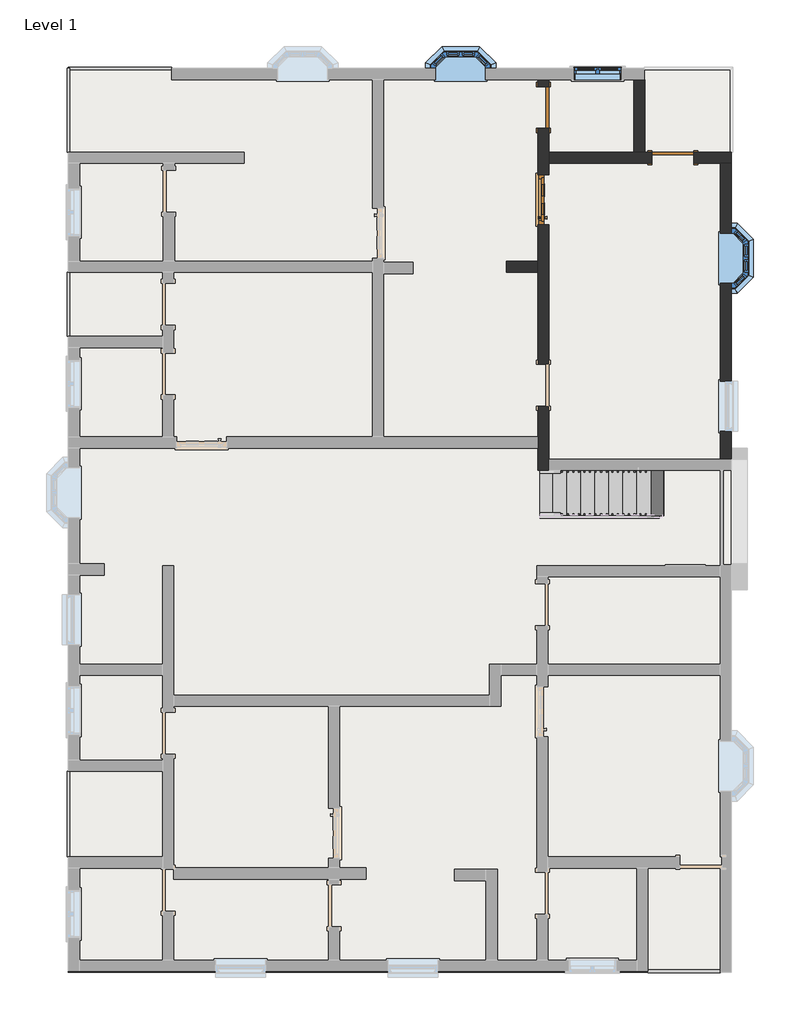
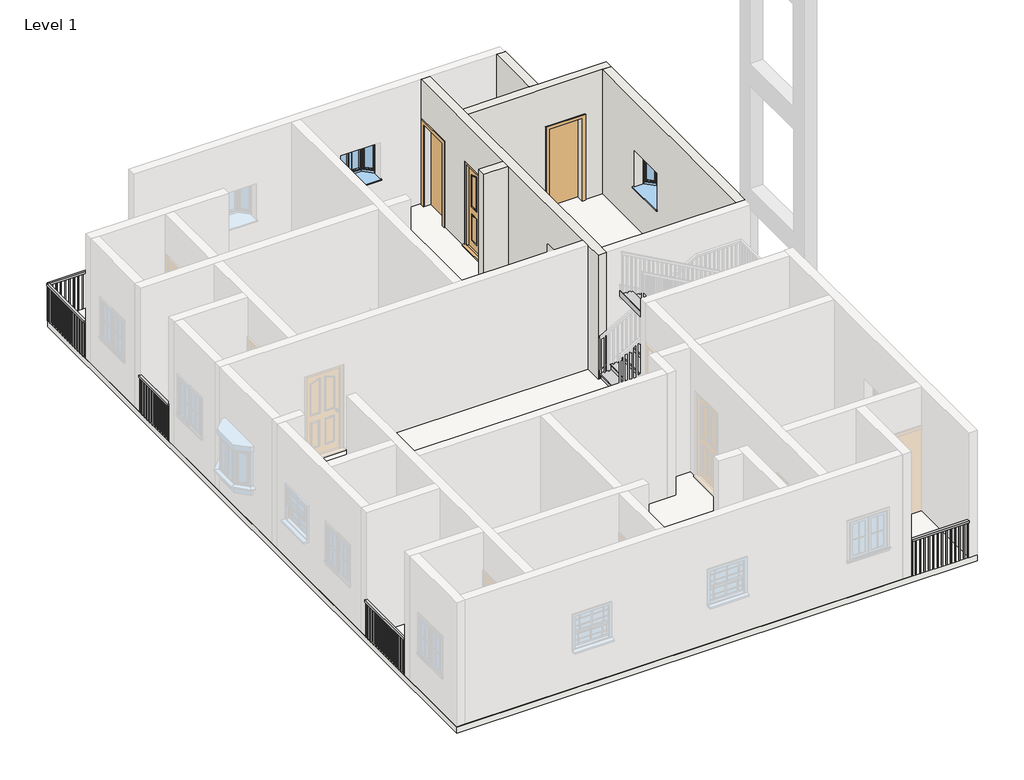
# One storey, part 2 of 4: 5 railings, 5 walls, 3 doors, 3 windows, 1 slab, 1 stair flight.
"""IFC4 building model written with IfcOpenShell, lengths in millimetres."""

from ifc_helpers import new_model, si_unit, frame, origin, origin_with_axes, place, context, project, spatial, polyline, outline, extrude, faceted_brep, transform, mapped, element, save
from components import doors_extsgl_12_910x2110mm_9a09825e, door_53b1b562, stair_flight_00d6430a, window_910x910mm_67ef725a, window_c29befe5

model = new_model("IFC4")

# Units and contexts
model_context = context("Model", 3, world=origin())
ifc_project = project(units=[si_unit("LENGTHUNIT", "METRE", prefix="MILLI")], contexts=[model_context])

# Site, building, storey
site = spatial("IfcSite", under=ifc_project)
building = spatial("IfcBuilding", under=site)
storey = spatial("IfcBuildingStorey", under=building, Name="Level 1", Elevation=0.0)

# Doors
placement = place(None, origin())
doors_extsgl_12_910x2110mm_shape = doors_extsgl_12_910x2110mm_9a09825e(model_context)
element("IfcDoor", 1, ObjectType="Doors_ExtSgl_12 : 910x2110mm", at=placement, inside=storey, context=model_context, shape_type="MappedRepresentation", body=[
    mapped(doors_extsgl_12_910x2110mm_shape, transform((1600.6941283, 5934.0547293, 0.0), x_axis=(0.0, 1.0, 0.0), y_axis=(-1.0, 0.0, 0.0), z_axis=(0.0, 0.0, 1.0))),
])
door_shape = door_53b1b562(model_context)
element("IfcDoor", 2, ObjectType="Single-Flush : 30\" x 80\"", at=placement, inside=storey, context=model_context, shape_type="MappedRepresentation", body=[
    mapped(door_shape, transform((1600.6941283, 7610.4547293, 0.0), x_axis=(0.0, 1.0, 0.0), y_axis=(-1.0, 0.0, 0.0), z_axis=(0.0, 0.0, 1.0))),
])
element("IfcDoor", 3, ObjectType="Single-Flush : 30\" x 80\"", at=placement, inside=storey, context=model_context, shape_type="MappedRepresentation", body=[
    mapped(door_shape, transform((3962.8941283, 6696.0547293, 0.0), x_axis=(-1.0, 0.0, 0.0), y_axis=(0.0, -1.0, 0.0), z_axis=(0.0, 0.0, 1.0))),
])

# Railings
element("IfcRailing", 4, ObjectType="Handrail - Rectangular", at=placement, inside=storey, context=model_context, shape_type="SweptSolid", body=[
    extrude(outline(polyline([(-7073.4058717, 4609.0339901), (-7022.6058717, 4609.0339901), (-7022.6058717, 3444.8547293), (-7073.4058717, 3444.8547293), (-7073.4058717, 4609.0339901)])), frame((0.0, 0.0, 863.6), z_axis=(0.0, 0.0, 1.0), x_axis=(1.0, 0.0, 0.0)), (0.0, 0.0, 1.0), 50.8),
    extrude(outline(polyline([(-7057.5308717, 3500.9589901), (-7038.4808717, 3500.9589901), (-7038.4808717, 3481.9089901), (-7057.5308717, 3481.9089901), (-7057.5308717, 3500.9589901)])), origin_with_axes(), (0.0, 0.0, 1.0), 863.6),
    extrude(outline(polyline([(-7057.5308717, 3602.5589901), (-7038.4808717, 3602.5589901), (-7038.4808717, 3583.5089901), (-7057.5308717, 3583.5089901), (-7057.5308717, 3602.5589901)])), origin_with_axes(), (0.0, 0.0, 1.0), 863.6),
    extrude(outline(polyline([(-7057.5308717, 3704.1589901), (-7038.4808717, 3704.1589901), (-7038.4808717, 3685.1089901), (-7057.5308717, 3685.1089901), (-7057.5308717, 3704.1589901)])), origin_with_axes(), (0.0, 0.0, 1.0), 863.6),
    extrude(outline(polyline([(-7057.5308717, 3805.7589901), (-7038.4808717, 3805.7589901), (-7038.4808717, 3786.7089901), (-7057.5308717, 3786.7089901), (-7057.5308717, 3805.7589901)])), origin_with_axes(), (0.0, 0.0, 1.0), 863.6),
    extrude(outline(polyline([(-7057.5308717, 3907.3589901), (-7038.4808717, 3907.3589901), (-7038.4808717, 3888.3089901), (-7057.5308717, 3888.3089901), (-7057.5308717, 3907.3589901)])), origin_with_axes(), (0.0, 0.0, 1.0), 863.6),
    extrude(outline(polyline([(-7057.5308717, 4008.9589901), (-7038.4808717, 4008.9589901), (-7038.4808717, 3989.9089901), (-7057.5308717, 3989.9089901), (-7057.5308717, 4008.9589901)])), origin_with_axes(), (0.0, 0.0, 1.0), 863.6),
    extrude(outline(polyline([(-7057.5308717, 4110.5589901), (-7038.4808717, 4110.5589901), (-7038.4808717, 4091.5089901), (-7057.5308717, 4091.5089901), (-7057.5308717, 4110.5589901)])), origin_with_axes(), (0.0, 0.0, 1.0), 863.6),
    extrude(outline(polyline([(-7057.5308717, 4212.1589901), (-7038.4808717, 4212.1589901), (-7038.4808717, 4193.1089901), (-7057.5308717, 4193.1089901), (-7057.5308717, 4212.1589901)])), origin_with_axes(), (0.0, 0.0, 1.0), 863.6),
    extrude(outline(polyline([(-7057.5308717, 4313.7589901), (-7038.4808717, 4313.7589901), (-7038.4808717, 4294.7089901), (-7057.5308717, 4294.7089901), (-7057.5308717, 4313.7589901)])), origin_with_axes(), (0.0, 0.0, 1.0), 863.6),
    extrude(outline(polyline([(-7057.5308717, 4415.3589901), (-7038.4808717, 4415.3589901), (-7038.4808717, 4396.3089901), (-7057.5308717, 4396.3089901), (-7057.5308717, 4415.3589901)])), origin_with_axes(), (0.0, 0.0, 1.0), 863.6),
    extrude(outline(polyline([(-7057.5308717, 4516.9589901), (-7038.4808717, 4516.9589901), (-7038.4808717, 4497.9089901), (-7057.5308717, 4497.9089901), (-7057.5308717, 4516.9589901)])), origin_with_axes(), (0.0, 0.0, 1.0), 863.6),
    extrude(outline(polyline([(-7057.5308717, 3463.9047293), (-7038.4808717, 3463.9047293), (-7038.4808717, 3444.8547293), (-7057.5308717, 3444.8547293), (-7057.5308717, 3463.9047293)])), origin_with_axes(), (0.0, 0.0, 1.0), 863.6),
    extrude(outline(polyline([(-7057.5308717, 4609.0339901), (-7038.4808717, 4609.0339901), (-7038.4808717, 4589.9839901), (-7057.5308717, 4589.9839901), (-7057.5308717, 4609.0339901)])), origin_with_axes(), (0.0, 0.0, 1.0), 863.6),
])
element("IfcRailing", 5, ObjectType="Handrail - Rectangular", at=placement, inside=storey, context=model_context, shape_type="SweptSolid", body=[
    extrude(outline(polyline([(-7073.4058717, -4474.6886333), (-7022.6058717, -4474.6886333), (-7022.6058717, -6029.3452707), (-7073.4058717, -6029.3452707), (-7073.4058717, -4474.6886333)])), frame((0.0, 0.0, 863.6), z_axis=(0.0, 0.0, 1.0), x_axis=(1.0, 0.0, 0.0)), (0.0, 0.0, 1.0), 50.8),
    extrude(outline(polyline([(-7057.5308717, -5989.1636333), (-7038.4808717, -5989.1636333), (-7038.4808717, -6008.2136333), (-7057.5308717, -6008.2136333), (-7057.5308717, -5989.1636333)])), origin_with_axes(), (0.0, 0.0, 1.0), 863.6),
    extrude(outline(polyline([(-7057.5308717, -5887.5636333), (-7038.4808717, -5887.5636333), (-7038.4808717, -5906.6136333), (-7057.5308717, -5906.6136333), (-7057.5308717, -5887.5636333)])), origin_with_axes(), (0.0, 0.0, 1.0), 863.6),
    extrude(outline(polyline([(-7057.5308717, -5785.9636333), (-7038.4808717, -5785.9636333), (-7038.4808717, -5805.0136333), (-7057.5308717, -5805.0136333), (-7057.5308717, -5785.9636333)])), origin_with_axes(), (0.0, 0.0, 1.0), 863.6),
    extrude(outline(polyline([(-7057.5308717, -5684.3636333), (-7038.4808717, -5684.3636333), (-7038.4808717, -5703.4136333), (-7057.5308717, -5703.4136333), (-7057.5308717, -5684.3636333)])), origin_with_axes(), (0.0, 0.0, 1.0), 863.6),
    extrude(outline(polyline([(-7057.5308717, -5582.7636333), (-7038.4808717, -5582.7636333), (-7038.4808717, -5601.8136333), (-7057.5308717, -5601.8136333), (-7057.5308717, -5582.7636333)])), origin_with_axes(), (0.0, 0.0, 1.0), 863.6),
    extrude(outline(polyline([(-7057.5308717, -5481.1636333), (-7038.4808717, -5481.1636333), (-7038.4808717, -5500.2136333), (-7057.5308717, -5500.2136333), (-7057.5308717, -5481.1636333)])), origin_with_axes(), (0.0, 0.0, 1.0), 863.6),
    extrude(outline(polyline([(-7057.5308717, -5379.5636333), (-7038.4808717, -5379.5636333), (-7038.4808717, -5398.6136333), (-7057.5308717, -5398.6136333), (-7057.5308717, -5379.5636333)])), origin_with_axes(), (0.0, 0.0, 1.0), 863.6),
    extrude(outline(polyline([(-7057.5308717, -5277.9636333), (-7038.4808717, -5277.9636333), (-7038.4808717, -5297.0136333), (-7057.5308717, -5297.0136333), (-7057.5308717, -5277.9636333)])), origin_with_axes(), (0.0, 0.0, 1.0), 863.6),
    extrude(outline(polyline([(-7057.5308717, -5176.3636333), (-7038.4808717, -5176.3636333), (-7038.4808717, -5195.4136333), (-7057.5308717, -5195.4136333), (-7057.5308717, -5176.3636333)])), origin_with_axes(), (0.0, 0.0, 1.0), 863.6),
    extrude(outline(polyline([(-7057.5308717, -5074.7636333), (-7038.4808717, -5074.7636333), (-7038.4808717, -5093.8136333), (-7057.5308717, -5093.8136333), (-7057.5308717, -5074.7636333)])), origin_with_axes(), (0.0, 0.0, 1.0), 863.6),
    extrude(outline(polyline([(-7057.5308717, -4973.1636333), (-7038.4808717, -4973.1636333), (-7038.4808717, -4992.2136333), (-7057.5308717, -4992.2136333), (-7057.5308717, -4973.1636333)])), origin_with_axes(), (0.0, 0.0, 1.0), 863.6),
    extrude(outline(polyline([(-7057.5308717, -4871.5636333), (-7038.4808717, -4871.5636333), (-7038.4808717, -4890.6136333), (-7057.5308717, -4890.6136333), (-7057.5308717, -4871.5636333)])), origin_with_axes(), (0.0, 0.0, 1.0), 863.6),
    extrude(outline(polyline([(-7057.5308717, -4769.9636333), (-7038.4808717, -4769.9636333), (-7038.4808717, -4789.0136333), (-7057.5308717, -4789.0136333), (-7057.5308717, -4769.9636333)])), origin_with_axes(), (0.0, 0.0, 1.0), 863.6),
    extrude(outline(polyline([(-7057.5308717, -4668.3636333), (-7038.4808717, -4668.3636333), (-7038.4808717, -4687.4136333), (-7057.5308717, -4687.4136333), (-7057.5308717, -4668.3636333)])), origin_with_axes(), (0.0, 0.0, 1.0), 863.6),
    extrude(outline(polyline([(-7057.5308717, -4566.7636333), (-7038.4808717, -4566.7636333), (-7038.4808717, -4585.8136333), (-7057.5308717, -4585.8136333), (-7057.5308717, -4566.7636333)])), origin_with_axes(), (0.0, 0.0, 1.0), 863.6),
    extrude(outline(polyline([(-7057.5308717, -6010.2952707), (-7038.4808717, -6010.2952707), (-7038.4808717, -6029.3452707), (-7057.5308717, -6029.3452707), (-7057.5308717, -6010.2952707)])), origin_with_axes(), (0.0, 0.0, 1.0), 863.6),
    extrude(outline(polyline([(-7057.5308717, -4474.6886333), (-7038.4808717, -4474.6886333), (-7038.4808717, -4493.7386333), (-7057.5308717, -4493.7386333), (-7057.5308717, -4474.6886333)])), origin_with_axes(), (0.0, 0.0, 1.0), 863.6),
])
element("IfcRailing", 6, ObjectType="Handrail - Rectangular", at=placement, inside=storey, context=model_context, shape_type="SweptSolid", body=[
    extrude(outline(polyline([(3505.6941283, -8137.5452707), (3505.6941283, -8086.7452707), (4826.4941283, -8086.7452707), (4826.4941283, -8137.5452707), (3505.6941283, -8137.5452707)])), frame((0.0, 0.0, 863.6), z_axis=(0.0, 0.0, 1.0), x_axis=(1.0, 0.0, 0.0)), (0.0, 0.0, 1.0), 50.8),
    extrude(outline(polyline([(4715.3691283, -8121.6702707), (4715.3691283, -8102.6202707), (4734.4191283, -8102.6202707), (4734.4191283, -8121.6702707), (4715.3691283, -8121.6702707)])), origin_with_axes(), (0.0, 0.0, 1.0), 863.6),
    extrude(outline(polyline([(4613.7691283, -8121.6702707), (4613.7691283, -8102.6202707), (4632.8191283, -8102.6202707), (4632.8191283, -8121.6702707), (4613.7691283, -8121.6702707)])), origin_with_axes(), (0.0, 0.0, 1.0), 863.6),
    extrude(outline(polyline([(4512.1691283, -8121.6702707), (4512.1691283, -8102.6202707), (4531.2191283, -8102.6202707), (4531.2191283, -8121.6702707), (4512.1691283, -8121.6702707)])), origin_with_axes(), (0.0, 0.0, 1.0), 863.6),
    extrude(outline(polyline([(4410.5691283, -8121.6702707), (4410.5691283, -8102.6202707), (4429.6191283, -8102.6202707), (4429.6191283, -8121.6702707), (4410.5691283, -8121.6702707)])), origin_with_axes(), (0.0, 0.0, 1.0), 863.6),
    extrude(outline(polyline([(4308.9691283, -8121.6702707), (4308.9691283, -8102.6202707), (4328.0191283, -8102.6202707), (4328.0191283, -8121.6702707), (4308.9691283, -8121.6702707)])), origin_with_axes(), (0.0, 0.0, 1.0), 863.6),
    extrude(outline(polyline([(4207.3691283, -8121.6702707), (4207.3691283, -8102.6202707), (4226.4191283, -8102.6202707), (4226.4191283, -8121.6702707), (4207.3691283, -8121.6702707)])), origin_with_axes(), (0.0, 0.0, 1.0), 863.6),
    extrude(outline(polyline([(4105.7691283, -8121.6702707), (4105.7691283, -8102.6202707), (4124.8191283, -8102.6202707), (4124.8191283, -8121.6702707), (4105.7691283, -8121.6702707)])), origin_with_axes(), (0.0, 0.0, 1.0), 863.6),
    extrude(outline(polyline([(4004.1691283, -8121.6702707), (4004.1691283, -8102.6202707), (4023.2191283, -8102.6202707), (4023.2191283, -8121.6702707), (4004.1691283, -8121.6702707)])), origin_with_axes(), (0.0, 0.0, 1.0), 863.6),
    extrude(outline(polyline([(3902.5691283, -8121.6702707), (3902.5691283, -8102.6202707), (3921.6191283, -8102.6202707), (3921.6191283, -8121.6702707), (3902.5691283, -8121.6702707)])), origin_with_axes(), (0.0, 0.0, 1.0), 863.6),
    extrude(outline(polyline([(3800.9691283, -8121.6702707), (3800.9691283, -8102.6202707), (3820.0191283, -8102.6202707), (3820.0191283, -8121.6702707), (3800.9691283, -8121.6702707)])), origin_with_axes(), (0.0, 0.0, 1.0), 863.6),
    extrude(outline(polyline([(3699.3691283, -8121.6702707), (3699.3691283, -8102.6202707), (3718.4191283, -8102.6202707), (3718.4191283, -8121.6702707), (3699.3691283, -8121.6702707)])), origin_with_axes(), (0.0, 0.0, 1.0), 863.6),
    extrude(outline(polyline([(3597.7691283, -8121.6702707), (3597.7691283, -8102.6202707), (3616.8191283, -8102.6202707), (3616.8191283, -8121.6702707), (3597.7691283, -8121.6702707)])), origin_with_axes(), (0.0, 0.0, 1.0), 863.6),
    extrude(outline(polyline([(4807.4441283, -8121.6702707), (4807.4441283, -8102.6202707), (4826.4941283, -8102.6202707), (4826.4941283, -8121.6702707), (4807.4441283, -8121.6702707)])), origin_with_axes(), (0.0, 0.0, 1.0), 863.6),
    extrude(outline(polyline([(3505.6941283, -8121.6702707), (3505.6941283, -8102.6202707), (3524.7441283, -8102.6202707), (3524.7441283, -8121.6702707), (3505.6941283, -8121.6702707)])), origin_with_axes(), (0.0, 0.0, 1.0), 863.6),
])
element("IfcRailing", 7, ObjectType="Handrail - Rectangular", at=placement, inside=storey, context=model_context, shape_type="SweptSolid", body=[
    extrude(outline(polyline([(-7022.6058717, 6797.6547293), (-7073.4058717, 6797.6547293), (-7073.4058717, 8321.6547293), (-7022.6058717, 8321.6547293), (-7022.6058717, 6797.6547293)])), frame((0.0, 0.0, 863.6), z_axis=(0.0, 0.0, 1.0), x_axis=(1.0, 0.0, 0.0)), (0.0, 0.0, 1.0), 50.8),
    extrude(outline(polyline([(-7038.4808717, 8210.5297293), (-7057.5308717, 8210.5297293), (-7057.5308717, 8229.5797293), (-7038.4808717, 8229.5797293), (-7038.4808717, 8210.5297293)])), origin_with_axes(), (0.0, 0.0, 1.0), 863.6),
    extrude(outline(polyline([(-7038.4808717, 8108.9297293), (-7057.5308717, 8108.9297293), (-7057.5308717, 8127.9797293), (-7038.4808717, 8127.9797293), (-7038.4808717, 8108.9297293)])), origin_with_axes(), (0.0, 0.0, 1.0), 863.6),
    extrude(outline(polyline([(-7038.4808717, 8007.3297293), (-7057.5308717, 8007.3297293), (-7057.5308717, 8026.3797293), (-7038.4808717, 8026.3797293), (-7038.4808717, 8007.3297293)])), origin_with_axes(), (0.0, 0.0, 1.0), 863.6),
    extrude(outline(polyline([(-7038.4808717, 7905.7297293), (-7057.5308717, 7905.7297293), (-7057.5308717, 7924.7797293), (-7038.4808717, 7924.7797293), (-7038.4808717, 7905.7297293)])), origin_with_axes(), (0.0, 0.0, 1.0), 863.6),
    extrude(outline(polyline([(-7038.4808717, 7804.1297293), (-7057.5308717, 7804.1297293), (-7057.5308717, 7823.1797293), (-7038.4808717, 7823.1797293), (-7038.4808717, 7804.1297293)])), origin_with_axes(), (0.0, 0.0, 1.0), 863.6),
    extrude(outline(polyline([(-7038.4808717, 7702.5297293), (-7057.5308717, 7702.5297293), (-7057.5308717, 7721.5797293), (-7038.4808717, 7721.5797293), (-7038.4808717, 7702.5297293)])), origin_with_axes(), (0.0, 0.0, 1.0), 863.6),
    extrude(outline(polyline([(-7038.4808717, 7600.9297293), (-7057.5308717, 7600.9297293), (-7057.5308717, 7619.9797293), (-7038.4808717, 7619.9797293), (-7038.4808717, 7600.9297293)])), origin_with_axes(), (0.0, 0.0, 1.0), 863.6),
    extrude(outline(polyline([(-7038.4808717, 7499.3297293), (-7057.5308717, 7499.3297293), (-7057.5308717, 7518.3797293), (-7038.4808717, 7518.3797293), (-7038.4808717, 7499.3297293)])), origin_with_axes(), (0.0, 0.0, 1.0), 863.6),
    extrude(outline(polyline([(-7038.4808717, 7397.7297293), (-7057.5308717, 7397.7297293), (-7057.5308717, 7416.7797293), (-7038.4808717, 7416.7797293), (-7038.4808717, 7397.7297293)])), origin_with_axes(), (0.0, 0.0, 1.0), 863.6),
    extrude(outline(polyline([(-7038.4808717, 7296.1297293), (-7057.5308717, 7296.1297293), (-7057.5308717, 7315.1797293), (-7038.4808717, 7315.1797293), (-7038.4808717, 7296.1297293)])), origin_with_axes(), (0.0, 0.0, 1.0), 863.6),
    extrude(outline(polyline([(-7038.4808717, 7194.5297293), (-7057.5308717, 7194.5297293), (-7057.5308717, 7213.5797293), (-7038.4808717, 7213.5797293), (-7038.4808717, 7194.5297293)])), origin_with_axes(), (0.0, 0.0, 1.0), 863.6),
    extrude(outline(polyline([(-7038.4808717, 7092.9297293), (-7057.5308717, 7092.9297293), (-7057.5308717, 7111.9797293), (-7038.4808717, 7111.9797293), (-7038.4808717, 7092.9297293)])), origin_with_axes(), (0.0, 0.0, 1.0), 863.6),
    extrude(outline(polyline([(-7038.4808717, 6991.3297293), (-7057.5308717, 6991.3297293), (-7057.5308717, 7010.3797293), (-7038.4808717, 7010.3797293), (-7038.4808717, 6991.3297293)])), origin_with_axes(), (0.0, 0.0, 1.0), 863.6),
    extrude(outline(polyline([(-7038.4808717, 6889.7297293), (-7057.5308717, 6889.7297293), (-7057.5308717, 6908.7797293), (-7038.4808717, 6908.7797293), (-7038.4808717, 6889.7297293)])), origin_with_axes(), (0.0, 0.0, 1.0), 863.6),
    extrude(outline(polyline([(-7038.4808717, 8302.6047293), (-7057.5308717, 8302.6047293), (-7057.5308717, 8321.6547293), (-7038.4808717, 8321.6547293), (-7038.4808717, 8302.6047293)])), origin_with_axes(), (0.0, 0.0, 1.0), 863.6),
    extrude(outline(polyline([(-7038.4808717, 6797.6547293), (-7057.5308717, 6797.6547293), (-7057.5308717, 6816.7047293), (-7038.4808717, 6816.7047293), (-7038.4808717, 6797.6547293)])), origin_with_axes(), (0.0, 0.0, 1.0), 863.6),
])
element("IfcRailing", 8, ObjectType="Handrail - Rectangular", at=placement, inside=storey, context=model_context, shape_type="SweptSolid", body=[
    extrude(outline(polyline([(-7048.0058717, 8296.2547293), (-7048.0058717, 8347.0547293), (-5168.4058717, 8347.0547293), (-5168.4058717, 8296.2547293), (-7048.0058717, 8296.2547293)])), frame((0.0, 0.0, 863.6), z_axis=(0.0, 0.0, 1.0), x_axis=(1.0, 0.0, 0.0)), (0.0, 0.0, 1.0), 50.8),
    extrude(outline(polyline([(-5228.7308717, 8312.1297293), (-5228.7308717, 8331.1797293), (-5209.6808717, 8331.1797293), (-5209.6808717, 8312.1297293), (-5228.7308717, 8312.1297293)])), origin_with_axes(), (0.0, 0.0, 1.0), 863.6),
    extrude(outline(polyline([(-5330.3308717, 8312.1297293), (-5330.3308717, 8331.1797293), (-5311.2808717, 8331.1797293), (-5311.2808717, 8312.1297293), (-5330.3308717, 8312.1297293)])), origin_with_axes(), (0.0, 0.0, 1.0), 863.6),
    extrude(outline(polyline([(-5431.9308717, 8312.1297293), (-5431.9308717, 8331.1797293), (-5412.8808717, 8331.1797293), (-5412.8808717, 8312.1297293), (-5431.9308717, 8312.1297293)])), origin_with_axes(), (0.0, 0.0, 1.0), 863.6),
    extrude(outline(polyline([(-5533.5308717, 8312.1297293), (-5533.5308717, 8331.1797293), (-5514.4808717, 8331.1797293), (-5514.4808717, 8312.1297293), (-5533.5308717, 8312.1297293)])), origin_with_axes(), (0.0, 0.0, 1.0), 863.6),
    extrude(outline(polyline([(-5635.1308717, 8312.1297293), (-5635.1308717, 8331.1797293), (-5616.0808717, 8331.1797293), (-5616.0808717, 8312.1297293), (-5635.1308717, 8312.1297293)])), origin_with_axes(), (0.0, 0.0, 1.0), 863.6),
    extrude(outline(polyline([(-5736.7308717, 8312.1297293), (-5736.7308717, 8331.1797293), (-5717.6808717, 8331.1797293), (-5717.6808717, 8312.1297293), (-5736.7308717, 8312.1297293)])), origin_with_axes(), (0.0, 0.0, 1.0), 863.6),
    extrude(outline(polyline([(-5838.3308717, 8312.1297293), (-5838.3308717, 8331.1797293), (-5819.2808717, 8331.1797293), (-5819.2808717, 8312.1297293), (-5838.3308717, 8312.1297293)])), origin_with_axes(), (0.0, 0.0, 1.0), 863.6),
    extrude(outline(polyline([(-5939.9308717, 8312.1297293), (-5939.9308717, 8331.1797293), (-5920.8808717, 8331.1797293), (-5920.8808717, 8312.1297293), (-5939.9308717, 8312.1297293)])), origin_with_axes(), (0.0, 0.0, 1.0), 863.6),
    extrude(outline(polyline([(-6041.5308717, 8312.1297293), (-6041.5308717, 8331.1797293), (-6022.4808717, 8331.1797293), (-6022.4808717, 8312.1297293), (-6041.5308717, 8312.1297293)])), origin_with_axes(), (0.0, 0.0, 1.0), 863.6),
    extrude(outline(polyline([(-6143.1308717, 8312.1297293), (-6143.1308717, 8331.1797293), (-6124.0808717, 8331.1797293), (-6124.0808717, 8312.1297293), (-6143.1308717, 8312.1297293)])), origin_with_axes(), (0.0, 0.0, 1.0), 863.6),
    extrude(outline(polyline([(-6244.7308717, 8312.1297293), (-6244.7308717, 8331.1797293), (-6225.6808717, 8331.1797293), (-6225.6808717, 8312.1297293), (-6244.7308717, 8312.1297293)])), origin_with_axes(), (0.0, 0.0, 1.0), 863.6),
    extrude(outline(polyline([(-6346.3308717, 8312.1297293), (-6346.3308717, 8331.1797293), (-6327.2808717, 8331.1797293), (-6327.2808717, 8312.1297293), (-6346.3308717, 8312.1297293)])), origin_with_axes(), (0.0, 0.0, 1.0), 863.6),
    extrude(outline(polyline([(-6447.9308717, 8312.1297293), (-6447.9308717, 8331.1797293), (-6428.8808717, 8331.1797293), (-6428.8808717, 8312.1297293), (-6447.9308717, 8312.1297293)])), origin_with_axes(), (0.0, 0.0, 1.0), 863.6),
    extrude(outline(polyline([(-6549.5308717, 8312.1297293), (-6549.5308717, 8331.1797293), (-6530.4808717, 8331.1797293), (-6530.4808717, 8312.1297293), (-6549.5308717, 8312.1297293)])), origin_with_axes(), (0.0, 0.0, 1.0), 863.6),
    extrude(outline(polyline([(-6651.1308717, 8312.1297293), (-6651.1308717, 8331.1797293), (-6632.0808717, 8331.1797293), (-6632.0808717, 8312.1297293), (-6651.1308717, 8312.1297293)])), origin_with_axes(), (0.0, 0.0, 1.0), 863.6),
    extrude(outline(polyline([(-6752.7308717, 8312.1297293), (-6752.7308717, 8331.1797293), (-6733.6808717, 8331.1797293), (-6733.6808717, 8312.1297293), (-6752.7308717, 8312.1297293)])), origin_with_axes(), (0.0, 0.0, 1.0), 863.6),
    extrude(outline(polyline([(-6854.3308717, 8312.1297293), (-6854.3308717, 8331.1797293), (-6835.2808717, 8331.1797293), (-6835.2808717, 8312.1297293), (-6854.3308717, 8312.1297293)])), origin_with_axes(), (0.0, 0.0, 1.0), 863.6),
    extrude(outline(polyline([(-6955.9308717, 8312.1297293), (-6955.9308717, 8331.1797293), (-6936.8808717, 8331.1797293), (-6936.8808717, 8312.1297293), (-6955.9308717, 8312.1297293)])), origin_with_axes(), (0.0, 0.0, 1.0), 863.6),
    extrude(outline(polyline([(-5187.4558717, 8312.1297293), (-5187.4558717, 8331.1797293), (-5168.4058717, 8331.1797293), (-5168.4058717, 8312.1297293), (-5187.4558717, 8312.1297293)])), origin_with_axes(), (0.0, 0.0, 1.0), 863.6),
    extrude(outline(polyline([(-7048.0058717, 8312.1297293), (-7048.0058717, 8331.1797293), (-7028.9558717, 8331.1797293), (-7028.9558717, 8312.1297293), (-7048.0058717, 8312.1297293)])), origin_with_axes(), (0.0, 0.0, 1.0), 863.6),
])

# Slab
element("IfcSlab", 9, ObjectType="Generic - 12\"", at=placement, inside=storey, context=model_context, shape_type="SweptSolid", body=[
    extrude(outline(polyline([(5029.6941283, 8321.6547293), (5029.6941283, -8124.8452707), (-7048.0058717, -8124.8452707), (-7048.0058717, 8321.6547293), (5029.6941283, 8321.6547293)])), frame((0.0, 0.0, -152.4), z_axis=(0.0, 0.0, 1.0), x_axis=(1.0, 0.0, 0.0)), (0.0, 0.0, 1.0), 152.4),
])

# Stair flight
stair_flight_shape = stair_flight_00d6430a(model_context)
element("IfcStairFlight", 10, ObjectType="2\" Tread 1\" Nosing 1/4\" Riser", at=placement, inside=storey, context=model_context, shape_type="MappedRepresentation", body=[
    mapped(stair_flight_shape, transform((0.0, 0.0, 0.0), x_axis=(1.0, 0.0, 0.0), y_axis=(0.0, 1.0, 0.0), z_axis=(0.0, 0.0, 1.0))),
])

# Walls
element("IfcWall", 11, ObjectType="Generic - 4.5\"", at=placement, inside=storey, context=model_context, shape_type="Brep", body=[
    faceted_brep([(1499.0941283, 8118.4547293, 0.0), (1499.0941283, 7991.4547293, 0.0), (1499.0941283, 7991.4547293, 2032.0), (1499.0941283, 7229.4547293, 2032.0), (1499.0941283, 7229.4547293, 0.0), (1499.0941283, 6389.0547293, 0.0), (1499.0941283, 6389.0547293, 2110.0), (1499.0941283, 5479.0547293, 2110.0), (1499.0941283, 5479.0547293, 0.0), (1499.0941283, 4812.2339901, 0.0), (1499.0941283, 4609.0339901, 0.0), (1499.0941283, 2936.8547293, 0.0), (1499.0941283, 2936.8547293, 2032.0), (1499.0941283, 2174.8547293, 2032.0), (1499.0941283, 2174.8547293, 0.0), (1499.0941283, 1616.0547293, 0.0), (1499.0941283, 1412.8547293, 0.0), (1499.0941283, 1006.4547293, 0.0), (1499.0941283, 1006.4547293, 3048.0), (1499.0941283, 1412.8547293, 3048.0), (1499.0941283, 1616.0547293, 3048.0), (1499.0941283, 4609.0339901, 3048.0), (1499.0941283, 4812.2339901, 3048.0), (1499.0941283, 8118.4547293, 3048.0), (1702.2941283, 7991.4547293, 2032.0), (1702.2941283, 7991.4547293, 0.0), (1702.2941283, 8118.4547293, 0.0), (1702.2941283, 8118.4547293, 3048.0), (1702.2941283, 6797.6547293, 3048.0), (1702.2941283, 6594.4547293, 3048.0), (1702.2941283, 1209.6547293, 3048.0), (1702.2941283, 1006.4547293, 3048.0), (1702.2941283, 1006.4547293, 0.0), (1702.2941283, 1209.6547293, 0.0), (1702.2941283, 2174.8547293, 0.0), (1702.2941283, 2174.8547293, 2032.0), (1702.2941283, 2936.8547293, 2032.0), (1702.2941283, 2936.8547293, 0.0), (1702.2941283, 5479.0547293, 0.0), (1702.2941283, 5479.0547293, 2110.0), (1702.2941283, 6389.0547293, 2110.0), (1702.2941283, 6389.0547293, 0.0), (1702.2941283, 6594.4547293, 0.0), (1702.2941283, 6797.6547293, 0.0), (1702.2941283, 7229.4547293, 0.0), (1702.2941283, 7229.4547293, 2032.0)], [[[0, 1, 2, 3, 4, 5, 6, 7, 8, 9, 10, 11, 12, 13, 14, 15, 16, 17, 18, 19, 20, 21, 22, 23]], [[24, 25, 26, 27, 28, 29, 30, 31, 32, 33, 34, 35, 36, 37, 38, 39, 40, 41, 42, 43, 44, 45]], [[38, 37, 11, 10, 9, 8]], [[34, 33, 32, 17, 16, 15, 14]], [[26, 25, 1, 0]], [[44, 43, 42, 41, 5, 4]], [[23, 22, 21, 20, 19, 18, 31, 30, 29, 28, 27]], [[0, 23, 27, 26]], [[18, 17, 32, 31]], [[8, 7, 39, 38]], [[6, 5, 41, 40]], [[7, 6, 40, 39]], [[12, 11, 37, 36]], [[13, 12, 36, 35]], [[14, 13, 35, 34]], [[2, 1, 25, 24]], [[3, 2, 24, 45]], [[4, 3, 45, 44]]]),
])
element("IfcWall", 12, ObjectType="Generic - 4.5\"", at=placement, inside=storey, context=model_context, shape_type="Brep", body=[
    faceted_brep([(1702.2941283, 6594.4547293, 0.0), (3581.8941283, 6594.4547293, 0.0), (3581.8941283, 6594.4547293, 2032.0), (4343.8941283, 6594.4547293, 2032.0), (4343.8941283, 6594.4547293, 0.0), (4826.4941283, 6594.4547293, 0.0), (5029.6941283, 6594.4547293, 0.0), (5029.6941283, 6594.4547293, 3048.0), (4826.4941283, 6594.4547293, 3048.0), (1702.2941283, 6594.4547293, 3048.0), (3581.8941283, 6797.6547293, 2032.0), (3581.8941283, 6797.6547293, 0.0), (3454.8941283, 6797.6547293, 0.0), (3251.6941283, 6797.6547293, 0.0), (1702.2941283, 6797.6547293, 0.0), (1702.2941283, 6797.6547293, 3048.0), (3251.6941283, 6797.6547293, 3048.0), (3454.8941283, 6797.6547293, 3048.0), (5029.6941283, 6797.6547293, 3048.0), (5029.6941283, 6797.6547293, 0.0), (4343.8941283, 6797.6547293, 0.0), (4343.8941283, 6797.6547293, 2032.0)], [[[0, 1, 2, 3, 4, 5, 6, 7, 8, 9]], [[10, 11, 12, 13, 14, 15, 16, 17, 18, 19, 20, 21]], [[20, 19, 6, 5, 4]], [[14, 13, 12, 11, 1, 0]], [[9, 8, 7, 18, 17, 16, 15]], [[0, 9, 15, 14]], [[2, 1, 11, 10]], [[3, 2, 10, 21]], [[4, 3, 21, 20]], [[7, 6, 19, 18]]]),
])
element("IfcWall", 13, ObjectType="Generic - 4.5\"", at=placement, inside=storey, context=model_context, shape_type="Brep", body=[
    faceted_brep([(3251.6941283, 8118.4547293, 0.0), (3251.6941283, 6797.6547293, 0.0), (3251.6941283, 6797.6547293, 3048.0), (3251.6941283, 8118.4547293, 3048.0), (3454.8941283, 8118.4547293, 0.0), (3454.8941283, 8118.4547293, 3048.0), (3454.8941283, 6797.6547293, 3048.0), (3454.8941283, 6797.6547293, 0.0), (3442.1941283, 8118.4547293, 0.0), (3442.1941283, 8118.4547293, 3048.0)], [[[0, 1, 2, 3]], [[4, 5, 6, 7]], [[1, 0, 8, 4, 7]], [[3, 2, 6, 5, 9]], [[0, 3, 9, 5, 4, 8]], [[2, 1, 7, 6]]]),
])
element("IfcWall", 14, ObjectType="Generic - 4.5\"", at=placement, inside=storey, context=model_context, shape_type="SweptSolid", body=[
    extrude(outline(polyline([(927.5941283, 4812.2339901), (1499.0941283, 4812.2339901), (1499.0941283, 4609.0339901), (927.5941283, 4609.0339901), (927.5941283, 4812.2339901)])), origin_with_axes(), (0.0, 0.0, 1.0), 3048.0),
])
element("IfcWall", 15, ObjectType="Generic - 9\"", at=placement, inside=storey, context=model_context, shape_type="SweptSolid", body=[
    extrude(outline(polyline([(6594.4547293, 0.0), (1209.6547293, 0.0), (1209.6547293, 3048.0), (6594.4547293, 3048.0), (6594.4547293, 0.0)]), holes=[polyline([(5322.2547293, 1824.4), (4412.2547293, 1824.4), (4412.2547293, 914.4), (5322.2547293, 914.4), (5322.2547293, 1824.4)]), polyline([(2629.8547293, 914.4), (2629.8547293, 1824.4), (1719.8547293, 1824.4), (1719.8547293, 914.4), (2629.8547293, 914.4)])]), frame((4826.4941283, 0.0, 0.0), z_axis=(1.0, 0.0, 0.0), x_axis=(0.0, 1.0, 0.0)), (0.0, 0.0, 1.0), 203.2),
])

# Windows
window_910x910mm_shape = window_910x910mm_67ef725a(model_context)
element("IfcWindow", 16, ObjectType="910x910mm", at=placement, inside=storey, context=model_context, shape_type="MappedRepresentation", body=[
    mapped(window_910x910mm_shape, transform((4919.6375605, 4297.2547293, -285.6), x_axis=(0.0, -1.0, 0.0), y_axis=(1.0, 0.0, 0.0), z_axis=(0.0, 0.0, 1.0))),
])
element("IfcWindow", 17, ObjectType="910x910mm", at=placement, inside=storey, context=model_context, shape_type="MappedRepresentation", body=[
    mapped(window_910x910mm_shape, transform((665.7441283, 8211.5981615, -285.6), x_axis=(1.0, 0.0, 0.0), y_axis=(0.0, 1.0, 0.0), z_axis=(0.0, 0.0, 1.0))),
])
window_shape = window_c29befe5(model_context)
element("IfcWindow", 18, ObjectType="Window-Casement-Double : 34\" x 36\"", at=placement, inside=storey, context=model_context, shape_type="MappedRepresentation", body=[
    mapped(window_shape, transform((2591.2941283, 8220.0547293, 0.0), x_axis=(1.0, 0.0, 0.0), y_axis=(0.0, 1.0, 0.0), z_axis=(0.0, 0.0, 1.0))),
])

save(model, "model.ifc")

# Revit data of these elements
# Type "Doors_ExtSgl_12 : 910x2110mm"
#   Type Mark = "10"
#   Type Comments = "External Single"
#   Operation = "SingleSwingRight"
#   Construction Type Id = "SGL"
#   Keynote = "L20"
#   Analytic Construction = "Large single-glazed windows"
#   Wrap Layers (Int) from Ext = 0' - 6.98819"
#   Wrap Layers (Ext) from Ext = 0' - 4.03543"
#   Visual Light Transmittance = 0.9
#   Thickness = 0' - 1.73228"
#   Stile Top of Lock rail = 3' - 3.37008"
#   Stile Top Rail = 0' - 5.90551"
#   Stile Shutting = 0' - 4.92126"
#   Stile Muntin Rail = 0' - 4.92126"
#   Stile Lock Rail = 0' - 6.88976"
#   Stile Hanging = 0' - 4.92126"
#   Stile Bottom Rail = 0' - 6.88976"
#   Solar Heat Gain Coefficient = 0.86
#   Rough Width = 2' - 11.82677"
#   Rough Height = 6' - 11.07087"
#   O/A Frame Width = 0' - 2.51969"
#   Heat Transfer Coefficient (U) = 0.979472 BTU/(h·ft²·°F)
#   Handle Z Distance = 3' - 3.37008"
#   Glazing Thickness = 0' - 0.94488"
#   FrameWidth = 0' - 1.65354"
#   FrameOffset - External = 0' - 0.98425"
#   FrameDepth = 0' - 3.50394"
#   Door Panel Width = 2' - 7.77165"
#   Door Panel Thickness = 0' - 1.73228"
#   Door Panel Height = 6' - 6.74016"
#   Cill Thickness = 0' - 2.14567"
#   Cill Projection = 0' - 1.1811"
#   Handle X Distance = 0' - 2.95276"
#   Height = 6' - 11.07087"
#   Structural Tolerance = 0' - 0.25591"
#   Tolerance = 0' - 0.11811"
#   Undercut = 0' - 0.15748"
#   Width = 2' - 11.82677"
#   Cill Extension = 0' - 0.98425"
#   Cavity Closer Width = 0' - 1.9685"
#   Cavity Closer Offset from Ext = 0' - 4.03543"
#   Cavity Closer Depth = 0' - 3.34646"
#   Vis - Ironmongery = yes
#   Vis - Cavity Closers = yes
#   Define Thermal Properties by = 1
#   Function = 1
#   Material Glass = Door - Glazing
#   Material Door = Door - Panel
#   Material Frame = Door - Frame/Mullion
#   Material Ironmongery = Door - Handle
#   Wall Closure = (empty or 0)
# Type "Single-Flush : 30\" x 80\""
#   Type Mark = "5"
#   Construction Type Id = "MDOOR"
#   Assembly Code = "C1020"
#   Analytic Construction = "Metal"
#   Thickness = 0' - 2"
#   Heat Transfer Coefficient (U) = 0.651978 BTU/(h·ft²·°F)
#   Height = 6' - 8"
#   Trim Projection Ext = 0' - 1"
#   Trim Projection Int = 0' - 1"
#   Trim Width = 0' - 3"
#   Width = 2' - 6"
#   Define Thermal Properties by = 1
#   Define Thermal Properties by = 1
#   Door Material = Door - Panel
#   Frame Material = Door - Frame
#   Visual Light Transmittance = 0
#   Solar Heat Gain Coefficient = 0
#   Function = (empty or 0)
#   Wall Closure = (empty or 0)
# Type "Handrail - Rectangular"
#   Assembly Code = "C2010400"
#   built-in parameter 1008612 = 0.0416667 (stored number, unit not read)
#   built-in parameter 1008611 = 0.0416667 (stored number, unit not read)
#   built-in parameter 1008609 = 0.333333 (stored number, unit not read)
#   built-in parameter 1008604 = 0.166667 (stored number, unit not read)
#   built-in parameter 1008603 = 0.166667 (stored number, unit not read)
#   Railing Height = 3' - 0"
#   built-in parameter 1008630 = 2
#   built-in parameter 1008610 = 2
#   built-in parameter 1008618 = Baluster - Square : 3/4"
# Type "Generic - 12\""
#   Assembly Code = "B1010"
#   Function = 0
#   Layers, outside or top first: 0' - 6" no material (function 1)
# Type "Generic - 4.5\""
#   Assembly Code = "B2010"
#   Layers, outside or top first: 0' - 8" no material (function 1)
# Type "Generic - 9\""
#   Assembly Code = "B2010"
#   Layers, outside or top first: 0' - 8" no material (function 1)
# Type "910x910mm"
#   Type Mark = "18"
#   Operation = "UserDefined"
#   Construction Type Id = "GSP4R"
#   Keynote = "L10"
#   Analytic Construction = "1/8 in Pilkington single glazing"
#   Wrap Layers (Ext) from Ext = 0' - 4.03543"
#   Wrap Layers (Int) from Ext = 0' - 6.98819"
#   Window Board Projection = 0' - 0.98425"
#   Window Board Extention = 0' - 0.98425"
#   Visual Light Transmittance = 0.9
#   Solar Heat Gain Coefficient = 0.78
#   Heat Transfer Coefficient (U) = 0.6496 BTU/(h·ft²·°F)
#   Glazing Thickness = 0' - 0.94488"
#   DONT CHANGE - Splay Width = 0' - 7.41997"
#   Rough Width = 2' - 11.82677"
#   Rough Height = 2' - 11.82677"
#   Roof Thickness = 0' - 4.92126"
#   Roof Overhang = 0' - 1.5748"
#   Plinth Thickness = 0' - 6.88976"
#   Height = 2' - 11.82677"
#   Width = 2' - 11.82677"
#   Frame Depth = 0' - 2.55906"
#   Default Head Height = 6' - 11.07087"
#   Cill Depth = 0' - 3.44488"
#   Cavity Closer Width = 0' - 1.9685"
#   Cavity Closer Offset from Ext = 0' - 4.03543"
#   Cavity Closer Depth = 0' - 3.34646"
#   Vis - Cavity Closers = yes
#   Define Thermal Properties by = 1
#   Material Trim = Window Frame
#   Material Glass = Glass
#   Material Frame = Window Frame
#   Manufacturer = ""
#   Wall Closure = (empty or 0)
# Type "Window-Casement-Double : 34\" x 36\""
#   Type Mark = "14"
#   Fire Rating = "0.5h"
#   Assembly Code = "B2020100"
#   Analytic Construction = "Double glazing - domestic"
#   Frame Extension [instance default] = 0' - 0 1/4"
#   Window Inset [instance default] = 0' - 0"
#   Wall Thickness [instance default] = 0' - 6"
#   Interior Wall Closure [instance default] = 0' - 2 1/4"
#   Half Width = 1' - 5"
#   Visual Light Transmittance = 0.81
#   Thermal Resistance (R) = 1.8146 (h·ft²·°F)/BTU
#   Solar Heat Gain Coefficient = 0.76
#   Rough Width = 2' - 10 1/2"
#   Rough Height = 3' - 0 1/2"
#   Height = 3' - 0"
#   Heat Transfer Coefficient (U) = 0.5511 BTU/(h·ft²·°F)
#   Exterior Wall Closure [instance default] = 0' - 1 1/4"
#   Extension Jamb [instance default] = 0' - 2 1/4"
#   Default Sill Height = 3' - 0"
#   Width = 2' - 10"
#   Define Thermal Properties by = 0
#   Muntin Visibility = yes
#   Interior Trim Visibility [instance default] = yes
#   Exterior Trim Visibility [instance default] = yes
#   Extension Jamb Visibility [instance default] = yes
#   Interior Trim Material = Wood - Stained
#   Muntin Pattern = Muntin Pattern_2x2 : Muntin Pattern_2x2
#   Interior Trim = Trim-Window-Interior-Flat : Picture Frame
#   Interior Frame Material = Wood - Stained
#   Glass Panel Material = Glass
#   Exterior Trim Material = Clad - White
#   Exterior Trim = Trim-Window-Exterior-Flat : with Sill
#   Exterior Frame Material = Clad - White
#   Wall Closure = (empty or 0)
# Element 1 (IfcDoor, "Doors_ExtSgl_12 : 910x2110mm")
#   Phase Created = New Construction
#   Materials on its faces: "Door - Panel", "Door - Handle", "Door - Frame/Mullion", "Door - Glazing"
# Elements 2, 3 (IfcDoor, "Single-Flush : 30\" x 80\"")
#   Phase Created = New Construction
#   Materials on its faces: "Door - Frame", "Door - Panel"
# Elements 4, 5, 6, 7, 8 (IfcRailing, "Handrail - Rectangular")
#   Phase Created = New Construction
# Element 9 (IfcSlab, "Generic - 12\"")
#   Height Offset From Level = 0' - 0"
#   Phase Created = New Construction
#   Materials on its faces: "Default Floor", "Parking Stripe", "Render Material 41-165-0"
# Element 10 (IfcStairFlight, "2\" Tread 1\" Nosing 1/4\" Riser")
#   Phase Created = New Construction
# Elements 11, 14 (IfcWall, "Generic - 4.5\"")
#   Top Offset = 0' - 0"
#   Base Offset = 0' - 0"
#   wall height = 10' - 0"
#   Phase Created = New Construction
#   Base Constraint = Level 1
#   Top Constraint = Level 2
#   Materials on its faces: "Default Wall"
# Element 12 (IfcWall, "Generic - 4.5\"")
#   Top Offset = 0' - 0"
#   Base Offset = 0' - 0"
#   wall height = 10' - 0"
#   Phase Created = New Construction
#   Base Constraint = Level 1
#   Top Constraint = Level 2
#   Materials on its faces: "Default Wall", "Parking Stripe", "Door - Frame/Mullion"
# Element 13 (IfcWall, "Generic - 4.5\"")
#   Top Offset = 0' - 0"
#   Base Offset = 0' - 0"
#   wall height = 10' - 0"
#   Phase Created = New Construction
#   Base Constraint = Level 1
#   Top Constraint = Level 2
#   Materials on its faces: "Default Wall", "Parking Stripe"
# Element 15 (IfcWall, "Generic - 9\"")
#   Top Offset = 0' - 0"
#   Base Offset = 0' - 0"
#   wall height = 10' - 0"
#   Phase Created = New Construction
#   Base Constraint = Level 1
#   Top Constraint = Level 2
#   Materials on its faces: "Default Wall", "Door - Frame/Mullion"
# Element 16 (IfcWindow, "910x910mm")
#   Mark = "2"
#   Phase Created = New Construction
#   Materials on its faces: "Window Frame", "Glass"
# Element 17 (IfcWindow, "910x910mm")
#   Mark = "3"
#   Phase Created = New Construction
#   Materials on its faces: "Window Frame", "Glass"
# Element 18 (IfcWindow, "Window-Casement-Double : 34\" x 36\"")
#   Mark = "12"
#   Window Inset = 0' - 0"
#   Interior Wall Closure = 0' - 2 1/4"
#   Frame Extension = 0' - 0 1/4"
#   Exterior Wall Closure = 0' - 1 1/4"
#   Interior Trim Visibility = yes
#   Exterior Trim Visibility = yes
#   Phase Created = New Construction
#   Materials on its faces: "Wood - Stained", "Glass", "Clad - White"
# Materials
#   "Door - Glazing": colour RGB 0 0 255, transparency 0.75
#   "Door - Panel": class "Wood", colour RGB 210 159 95, transparency 0, Cost = 0
#   "Door - Frame/Mullion": class "Wood", colour RGB 212 179 113, transparency 0
#   "Door - Handle": colour RGB 247 247 247, transparency 0
#   "Door - Frame": colour RGB 118 70 51, transparency 0, Cost = 0
#   "Window Frame": colour RGB 249 249 249, transparency 0
#   "Glass": class "Glass", colour RGB 0 128 192, transparency 0.75, Description = "Soda Lime Glass", Cost = 0
#   "Wood - Stained": class "Wood", colour RGB 224 178 126, transparency 0, Cost = 0
#   "Clad - White": class "Wood", colour RGB 242 242 238, transparency 0, Cost = 0
#   "Default Floor": colour RGB 128 128 128, transparency 0, Cost = 0
#   "Parking Stripe": class "Paint", colour RGB 250 250 91, transparency 0, Cost = 0
#   "Render Material 41-165-0": colour RGB 41 165 0, transparency 0
#   "Default Wall": colour RGB 128 128 128, transparency 0, Cost = 0
